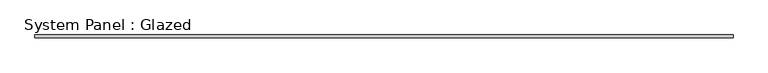
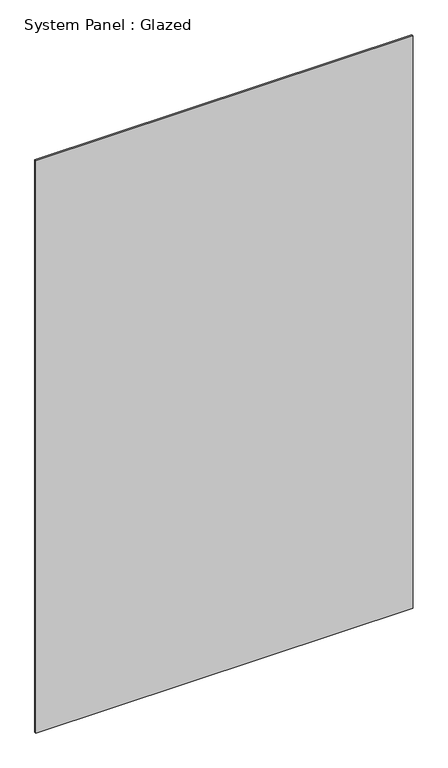
"""IFC4 building model written with IfcOpenShell, lengths in millimetres: plate geometry, System Panel : Glazed."""

from ifc_helpers import new_model, si_unit, origin, origin_with_axes, place, context, project, spatial, polyline, outline, extrude, source, transform, mapped, element, save


def system_panel_glazed_def3cda3(model_context):
    return source(origin(), model_context, "Body", "SweptSolid", [
        extrude(outline(polyline([(733.3333332, 34.0), (-733.3333332, 34.0), (-733.3333332, 40.0), (733.3333332, 40.0), (733.3333332, 34.0)])), origin_with_axes(), (0.0, 0.0, 1.0), 2350.0),
    ])


if __name__ == "__main__":
    model = new_model("IFC4")
    model_context = context("Model", 3, world=origin())
    ifc_project = project(units=[si_unit("LENGTHUNIT", "METRE", prefix="MILLI")], contexts=[model_context])
    site = spatial("IfcSite", under=ifc_project)
    building = spatial("IfcBuilding", under=site)
    placement = place(None, origin())
    system_panel_glazed_shape = system_panel_glazed_def3cda3(model_context)
    element("IfcPlate", 1, ObjectType="System Panel : Glazed", at=placement, inside=building, context=model_context, shape_type="MappedRepresentation", body=[
        mapped(system_panel_glazed_shape, transform((0.0, 0.0, 0.0), x_axis=(1.0, 0.0, 0.0), y_axis=(0.0, 1.0, 0.0), z_axis=(0.0, 0.0, 1.0))),
    ])
    save(model, "model.ifc")

# Revit data of these elements
# Type "System Panel : Glazed"
#   Construction Type Id = "GSP4R"
#   Analytic Construction = "1/8 in Pilkington single glazing"
#   Visual Light Transmittance = 0.9
#   Solar Heat Gain Coefficient = 0.86
#   Heat Transfer Coefficient (U) = 6.7069 W/(m²·K)
#   Define Thermal Properties by = 1
# Element 1 (IfcPlate, "System Panel : Glazed")
#   Materials on its faces: "Default New Material(6)"
# Materials
#   "Default New Material(6)": class "Generic", colour RGB 191 25 25, transparency 0.9, Cost = 0
